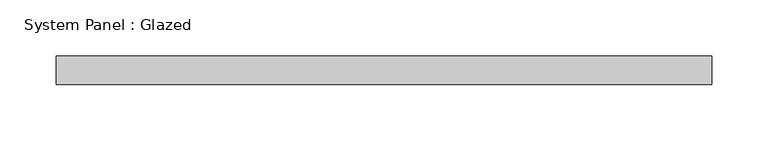
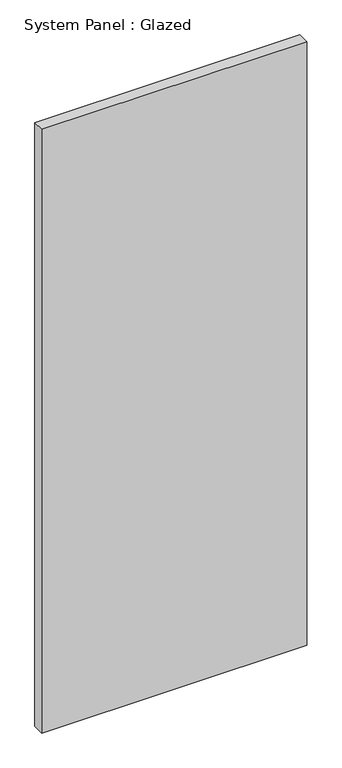
"""IFC4 building model written with IfcOpenShell, lengths in millimetres: plate geometry, System Panel : Glazed."""

from ifc_helpers import new_model, si_unit, origin, origin_with_axes, place, context, project, spatial, polyline, outline, extrude, source, transform, mapped, element, save


def system_panel_glazed_e283e605(model_context):
    return source(origin(), model_context, "Body", "SweptSolid", [
        extrude(outline(polyline([(290.9914477, 19.05), (-290.9914477, 19.05), (-290.9914477, 44.45), (290.9914477, 44.45), (290.9914477, 19.05)])), origin_with_axes(), (0.0, 0.0, 1.0), 1401.6649662),
    ])


if __name__ == "__main__":
    model = new_model("IFC4")
    model_context = context("Model", 3, world=origin())
    ifc_project = project(units=[si_unit("LENGTHUNIT", "METRE", prefix="MILLI")], contexts=[model_context])
    site = spatial("IfcSite", under=ifc_project)
    building = spatial("IfcBuilding", under=site)
    placement = place(None, origin())
    system_panel_glazed_shape = system_panel_glazed_e283e605(model_context)
    element("IfcPlate", 1, ObjectType="System Panel : Glazed", at=placement, inside=building, context=model_context, shape_type="MappedRepresentation", body=[
        mapped(system_panel_glazed_shape, transform((0.0, 0.0, 0.0), x_axis=(1.0, 0.0, 0.0), y_axis=(0.0, 1.0, 0.0), z_axis=(0.0, 0.0, 1.0))),
    ])
    save(model, "model.ifc")

# Revit data of these elements
# Type "System Panel : Glazed"
#   Construction Type Id = "GSP4R"
#   Analytic Construction = "1/8 in Pilkington single glazing"
#   Visual Light Transmittance = 0.9
#   Solar Heat Gain Coefficient = 0.86
#   Heat Transfer Coefficient (U) = 1.18115 BTU/(h·ft²·°F)
#   Define Thermal Properties by = 1
# Element 1 (IfcPlate, "System Panel : Glazed")
#   Materials on its faces: "Glass"
# Materials
#   "Glass": class "Glass", colour RGB 0 128 192, transparency 0.75, Description = "Soda Lime Glass", Cost = 0
